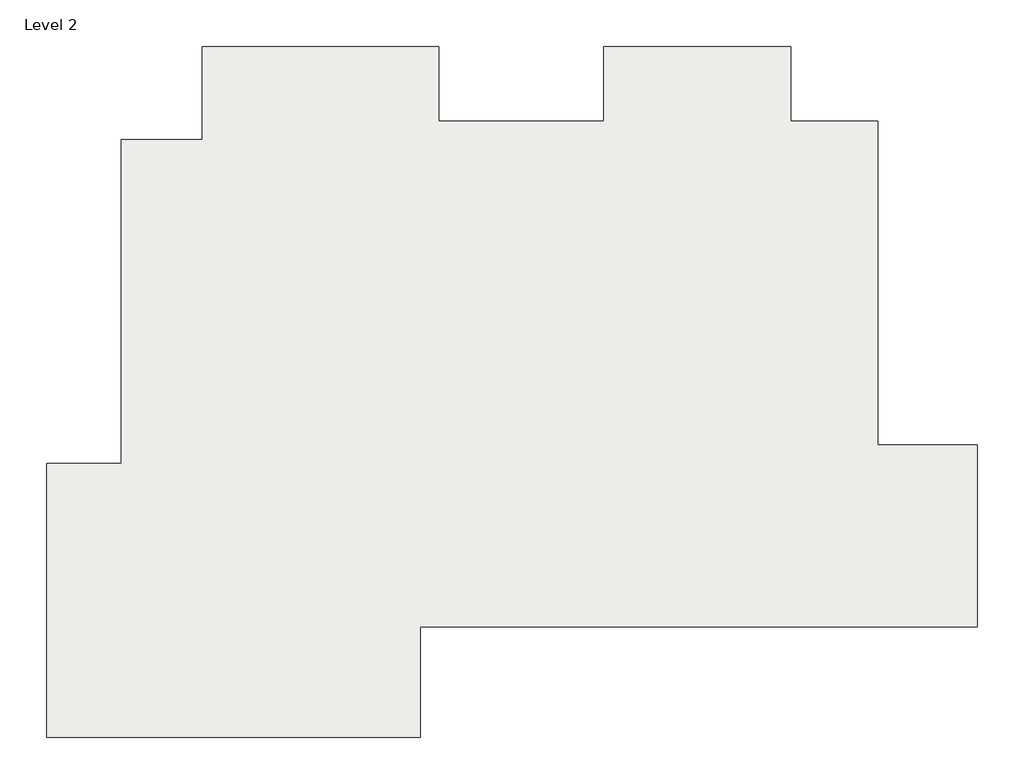
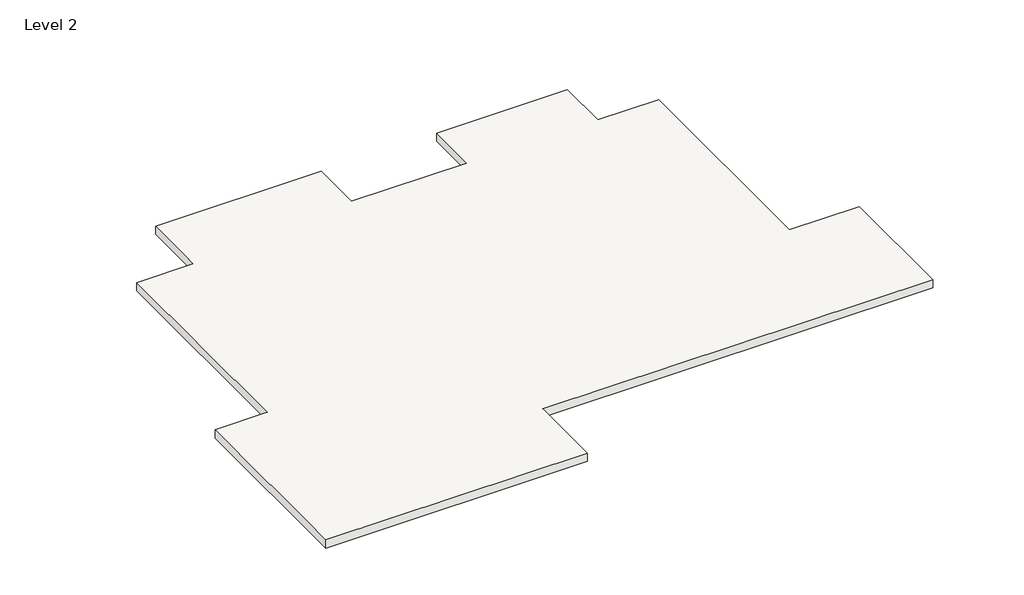
# One storey: 1 roof.
"""IFC4 building model written with IfcOpenShell, lengths in millimetres."""

from ifc_helpers import new_model, si_unit, frame, origin, place, context, project, spatial, polyline, outline, extrude, element, save

model = new_model("IFC4")

# Units and contexts
model_context = context("Model", 3, world=origin())
ifc_project = project(units=[si_unit("LENGTHUNIT", "METRE", prefix="MILLI")], contexts=[model_context])

# Site, building, storey
site = spatial("IfcSite", under=ifc_project)
building = spatial("IfcBuilding", under=site)
storey = spatial("IfcBuildingStorey", under=building, Name="Level 2", Elevation=3657.6)

# Roof
placement = place(None, origin())
element("IfcRoof", 1, ObjectType="6\" roof", at=placement, inside=storey, context=model_context, shape_type="SweptSolid", body=[
    extrude(outline(polyline([(-5221.9928023, 8045.1957931), (-5221.9928023, 9188.1957931), (-2326.3928023, 9188.1957931), (-2326.3928023, 8273.7957931), (-307.0928023, 8273.7957931), (-307.0928023, 9188.1957931), (1978.9071977, 9188.1957931), (1978.9071977, 8273.7957931), (3045.7071977, 8273.7957931), (3045.7071977, 4311.3957931), (4264.9071977, 4311.3957931), (4264.9071977, 2082.5457931), (-2554.9928023, 2082.5457931), (-2554.9928023, 729.9957931), (-7126.9928023, 729.9957931), (-7126.9928023, 4082.7957931), (-6212.5928023, 4082.7957931), (-6212.5928023, 8045.1957931), (-5221.9928023, 8045.1957931)])), frame((0.0, 0.0, 3657.6), z_axis=(0.0, 0.0, 1.0), x_axis=(1.0, 0.0, 0.0)), (0.0, 0.0, 1.0), 152.4),
])

save(model, "model.ifc")

# Revit data of these elements
# Type "6\" roof"
#   Assembly Code = "B1020"
#   Layers, outside or top first: 0' - 6" no material (function 1)
# Element 1 (IfcRoof, "6\" roof")
#   built-in parameter 1001705 = 12.5 (stored number, unit not read)
#   built-in parameter 1001710 = 33615
#   Phase Created = New Construction
#   Materials on its faces: "Default Roof"
# Materials
#   "Default Roof": colour RGB 88 101 114, transparency 0, Cost = 0
